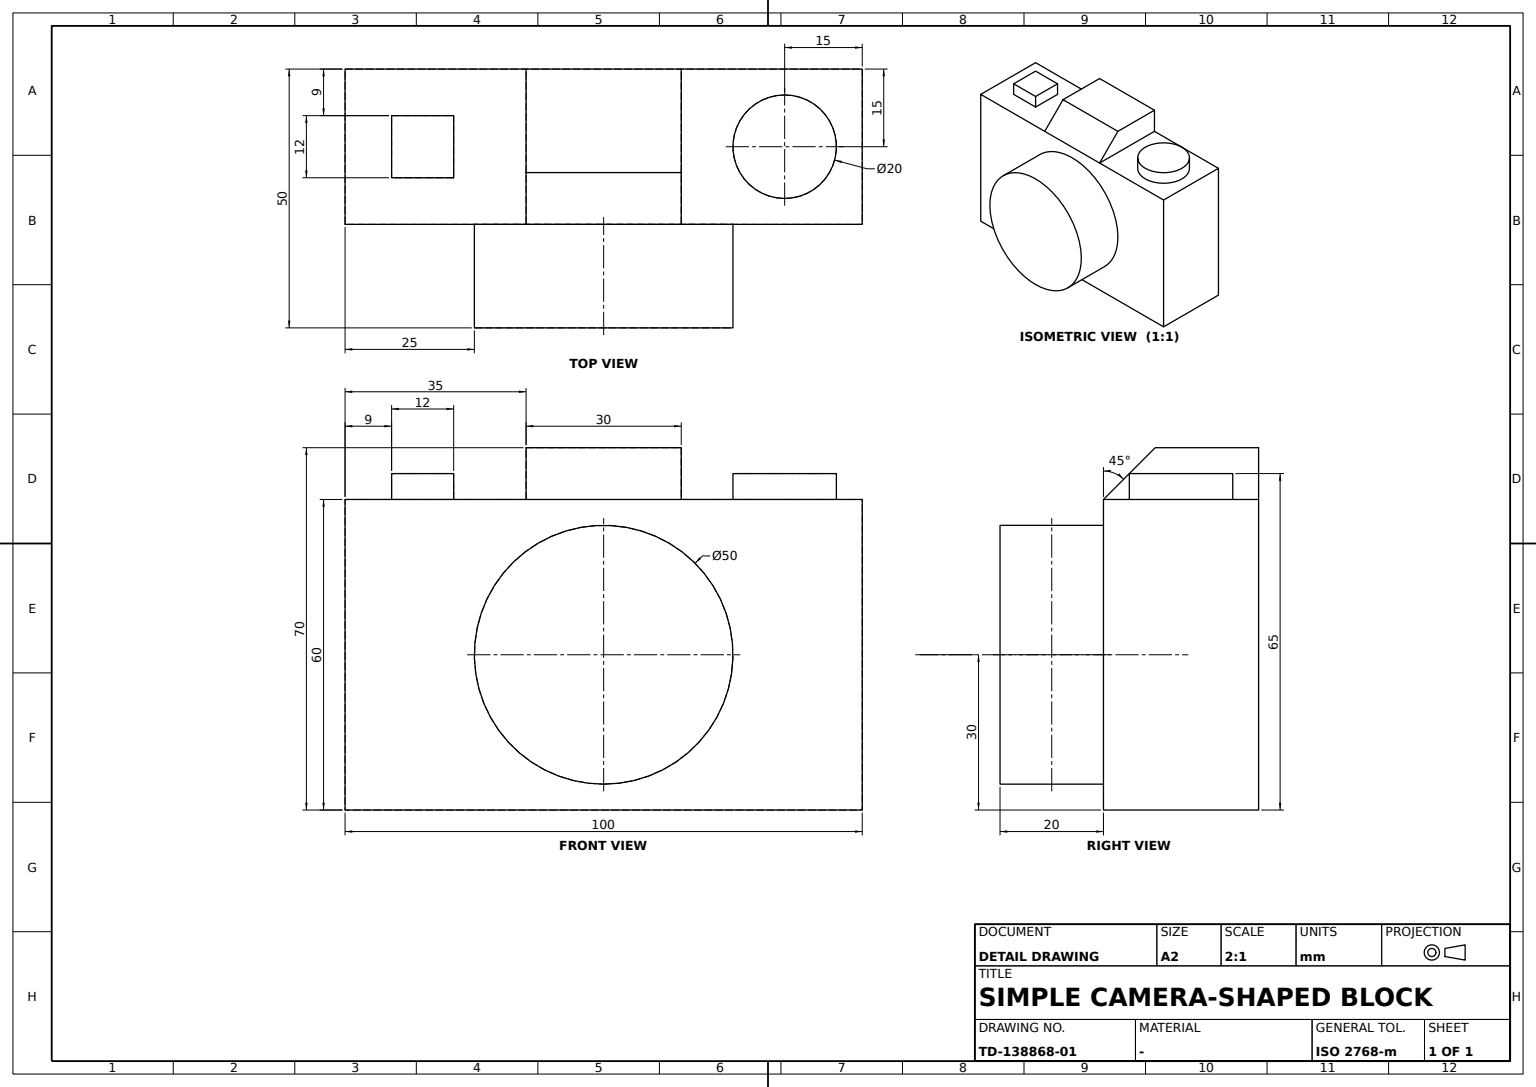
CATIA V5 part; units mm, degrees
sketch "Sketch1" plane through (0, 0, 0) normal (1, 0, 0) x (0, 1, 0)
  line L0 (50, 30) -> (50, -30)
  line L1 (50, -30) -> (-50, -30)
  line L2 (-50, -30) -> (-50, 30)
  line L3 (-50, 30) -> (50, 30)
  dimension "length L1" = 100
  dimension "length L0" = 60
  constraint vertical L0 y-axis
  constraint vertical L2 y-axis
  constraint horizontal L1 x-axis
  constraint horizontal L3 x-axis
  constraint equidistance L0 L2 origin
  constraint equidistance L1 L3 origin
extrude "Pad1" add sketch "Sketch1" along normal mid plane 30
sketch "Sketch2" plane through (15, 0, 0) normal (1, 0, 0) x (0, 1, 0)
  circle A0 centre (0, 0) radius 25
  dimension "radius A0" = 25
extrude "Pad2" add sketch "Sketch2" along normal blind 20
sketch "Sketch3" plane through (0, 0, 0) normal (0, 1, 0) x (-1, 0, 0)
  line L0 (-15, 30) -> (15, 30)
  line L1 (15, 30) -> (15, 40)
  line L2 (15, 40) -> (-5, 40)
  line L3 (-5, 40) -> (-15, 30)
  line L4 (15, 30) -> (-15, 30) construction
  line L5 (15, -30) -> (15, 30) construction
  dimension "length L0" = 30
  dimension "length L1" = 10
  dimension "angle L3 L0" = 45
  constraint horizontal L0 x-axis
  constraint horizontal L2 x-axis
  constraint vertical L1 y-axis
  constraint coincidence L0 L4
  constraint coincidence L1 L5
extrude "Pad3" add sketch "Sketch3" along normal mid plane 30
sketch "Sketch4" plane through (0, 0, 30) normal (0, 0, 1) x (0, 1, 0)
  circle A0 centre (35, 0) radius 10
  point P0 (35, 0)
  point P1 (-35, 0)
  line L0 (-29, 6) -> (-29, -6)
  line L1 (-29, -6) -> (-41, -6)
  line L2 (-41, -6) -> (-41, 6)
  line L3 (-41, 6) -> (-29, 6)
  line L4 (50, -15) -> (-50, -15) construction
  line L5 (50, 15) -> (50, -15) construction
  line L6 (-50, 15) -> (-50, -15) construction
  dimension "radius A0" = 10
  dimension "distance L4 P0" = 15
  dimension "distance P0 L5" = 15
  dimension "length L2" = 12
  dimension "length L1" = 12
  dimension "distance L6 P1" = 15
  constraint coincidence P1 x-axis
  constraint vertical L0 y-axis
  constraint vertical L2 y-axis
  constraint horizontal L1 x-axis
  constraint horizontal L3 x-axis
  constraint equidistance L0 L2 P1
  constraint equidistance L1 L3 P1
extrude "Pad4" add sketch "Sketch4" along normal blind 5
